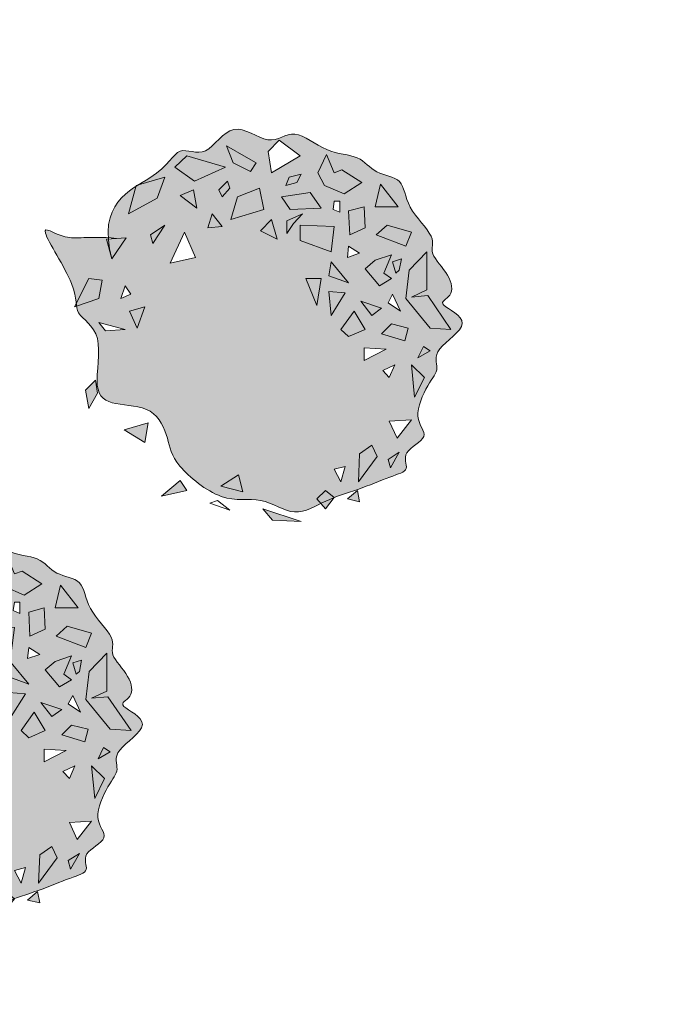
# Model space of a CAD drawing. Units: metres. Extents: x 4298.5 to 4325.2, y 2075 to 2095.8.
# Tile 24 of 35: x 4319.132 to 4320.125, y 2078.198 to 2079.73. Entities that reach past the tile are written whole.
import ezdxf

# ---------------------------------------------------------------- set-up
doc = ezdxf.new("R2010")
doc.units = ezdxf.units.M
doc.layers.add('A-ANNO-DIMS', color=2, linetype='Continuous', lineweight=18)
doc.layers.add('L-PLNT', color=94, linetype='Continuous', lineweight=13)
doc.layers.add('L-PLNT-PATT', color=116, linetype='Continuous', lineweight=13, true_color=0x13823e)
doc.styles.get("Standard").update_dxf_attribs({"font": 'arial.ttf'})
doc.dimstyles.get("Standard").update_dxf_attribs({"dimtxt": 0.18, "dimasz": 0.18, "dimexe": 0.18, "dimexo": 0.0625, "dimgap": 0.09, "dimtad": 0, "dimtih": 1, "dimtoh": 1, "dimdec": 4, "dimzin": 0, "dimdsep": 46, "dimtxsty": 'Standard', "dimcen": 0.09, "dimadec": 0, "dimazin": 0, "dimtfac": 1, "dimtdec": 4, "dimtofl": 0, "dimtmove": 0, "dimatfit": 3, "dimfxl": 1, "dimtolj": 1, "dimtzin": 0, "dimarcsym": 0})

# ---------------------------------------------------------------- blocks, each defined once
blk = doc.blocks.new('*U9')
for points in [[(-2.003, 11.656), (-1.598, 10.618), (-0.518, 10.099), (-0.181, 10.618), (-0.788, 10.964)], [(1.237, 12.003), (0.562, 11.31), (0.764, 10.013), (2.519, 11.051)], [(-4.432, 11.051), (-5.175, 10.359), (-3.96, 9.493), (-2.07, 10.359)], [(4.139, 11.137), (3.599, 10.013), (4.004, 9.234), (5.218, 8.715), (6.298, 9.407), (5.083, 10.186), (4.611, 10.013)], [(-5.782, 9.753), (-7.537, 9.234), (-8.009, 7.504), (-6.255, 8.455)], [(2.586, 9.926), (1.844, 9.753), (1.642, 9.234), (2.316, 9.407)], [(-1.935, 9.493), (-2.475, 8.974), (-2.273, 8.542), (-1.8, 9.061)], [(0.022, 9.061), (-1.328, 8.542), (-1.733, 7.157), (0.292, 7.763)], [(7.446, 9.32), (7.108, 7.936), (8.525, 7.936)], [(-4.837, 8.628), (-3.825, 7.85), (-4.027, 8.974)], [(1.372, 8.542), (3.126, 8.801), (3.801, 7.85), (1.912, 7.763)], [(4.611, 8.282), (4.544, 7.763), (4.949, 7.59), (4.949, 8.282)], [(6.433, 7.936), (5.488, 7.676), (5.556, 6.206), (6.501, 6.638)], [(-2.88, 7.504), (-3.15, 6.638), (-2.273, 6.725)], [(1.709, 6.292), (1.709, 7.071), (2.654, 7.504), (2.114, 6.898)], [(-5.782, 6.811), (-6.659, 6.206), (-6.524, 5.687)], [(0.764, 7.157), (0.089, 6.465), (1.102, 5.946)], [(2.519, 6.811), (2.519, 5.86), (4.409, 5.167), (4.611, 6.725)], [(7.851, 6.811), (7.176, 6.206), (8.998, 5.514), (9.335, 6.379)], [(-4.567, 6.379), (-5.445, 4.475), (-3.892, 4.821)], [(-8.144, 6.033), (-9.359, 5.946), (-9.022, 4.735)], [(5.488, 5.514), (5.421, 4.821), (6.163, 5.081)], [(8.12, 4.994), (7.108, 4.648), (6.501, 4.129), (7.378, 3.091), (8.12, 3.524), (7.648, 3.87)], [(10.28, 5.167), (9.2, 4.043), (8.998, 2.312), (10.482, 0.495), (11.765, 0.409), (10.348, 2.485), (9.335, 2.399), (10.28, 2.831)], [(4.409, 4.562), (4.274, 3.697), (5.488, 3.264)], [(8.728, 4.735), (8.188, 4.562), (8.39, 3.87), (8.593, 4.043)], [(-11.316, 1.793), (-9.831, 2.312), (-9.629, 3.437), (-10.439, 3.524)], [(-8.212, 3.091), (-8.482, 2.312), (-7.874, 2.572)], [(3.531, 1.88), (2.856, 3.524), (3.801, 3.524)], [(4.274, 2.745), (5.286, 2.658), (4.409, 1.274)], [(8.188, 2.572), (7.918, 2.053), (8.66, 1.534)], [(7.513, 1.707), (6.906, 1.274), (6.231, 2.139)], [(-6.997, 1.793), (-7.942, 1.534), (-7.469, 0.495)], [(5.826, 1.534), (5.016, 0.409), (5.488, -0.024), (6.501, 0.409)], [(-8.212, 0.409), (-9.426, 0.322), (-9.831, 0.841)], [(8.12, 0.755), (7.513, 0.149), (8.93, -0.283), (9.133, 0.495)], [(7.783, -0.803), (6.433, -1.495), (6.433, -0.716)], [(10.078, -0.629), (9.74, -1.322), (10.482, -0.889)], [(8.323, -1.754), (7.985, -2.533), (7.581, -2.1)], [(9.335, -1.754), (9.538, -3.744), (10.145, -2.533)], [(-10.034, -2.706), (-10.641, -3.312), (-10.439, -4.436), (-9.899, -3.485)], [(-8.279, -5.734), (-6.794, -5.302), (-6.997, -6.513)], [(9.335, -5.129), (8.458, -6.253), (7.985, -5.215)], [(6.096, -8.935), (6.163, -7.205), (6.906, -6.686), (7.243, -7.378)], [(8.053, -8.07), (8.593, -7.118), (7.918, -7.551)], [(5.286, -7.984), (4.611, -8.157), (5.016, -8.935)], [(-4.837, -8.849), (-4.432, -9.454), (-5.985, -9.801)], [(-2.34, -9.195), (-1.26, -8.503), (-0.99, -9.541)], [(4.071, -9.454), (3.531, -9.974), (4.071, -10.579), (4.611, -9.887)], [(6.028, -9.454), (5.421, -9.974), (6.163, -10.147)], [(-2.543, -10.06), (-3.015, -10.233), (-1.8, -10.666)], [(0.224, -10.579), (0.832, -11.272), (2.586, -11.358)]]:
    blk.add_lwpolyline(points, close=True)
blk = doc.blocks.new('*D47')
at = {"layer": 'A-ANNO-DIMS', "color": 0, "lineweight": -2, "transparency": 16777216}
for p, q in [((4300.4306, 2084.4956), (4300.4306, 2074.9896)), ((4322.8106, 2084.4956), (4322.8106, 2074.9896)), ((4300.6106, 2075.1696), (4311.2252, 2075.1696)), ((4322.6306, 2075.1696), (4312.016, 2075.1696))]:
    blk.add_line(p, q, dxfattribs=at)
at = {"layer": 'A-ANNO-DIMS', "color": 0, "transparency": 16777216}
for points in [[(4300.6106, 2075.1996), (4300.6106, 2075.1396), (4300.4306, 2075.1696)], [(4322.6306, 2075.1996), (4322.6306, 2075.1396), (4322.8106, 2075.1696)]]:
    blk.add_solid(points, dxfattribs=at)
at = {"layer": 'Defpoints', "color": 0, "transparency": 16777216}
for p in [(4300.4306, 2084.5581), (4322.8106, 2084.5581), (4322.8106, 2075.1696)]:
    blk.add_point(p, dxfattribs=at)
at = {"layer": 'A-ANNO-DIMS', "color": 0, "transparency": 16777216, "insert": (4311.6206, 2075.1696), "char_height": 0.18, "attachment_point": 5}
blk.add_mtext('\\A1;22.38', dxfattribs=at)
blk = doc.blocks.new('*D48')
at = {"layer": 'A-ANNO-DIMS', "color": 0, "lineweight": -2, "transparency": 16777216}
for p, q in [((4310.1831, 2094.4781), (4324.7671, 2094.4781)), ((4324.5871, 2094.2981), (4324.5871, 2085.585)), ((4324.5871, 2076.5081), (4324.5871, 2085.2212)), ((4316.8731, 2076.3281), (4324.7671, 2076.3281))]:
    blk.add_line(p, q, dxfattribs=at)
at = {"layer": 'A-ANNO-DIMS', "color": 0, "transparency": 16777216}
for points in [[(4324.5571, 2094.2981), (4324.6171, 2094.2981), (4324.5871, 2094.4781)], [(4324.5571, 2076.5081), (4324.6171, 2076.5081), (4324.5871, 2076.3281)]]:
    blk.add_solid(points, dxfattribs=at)
at = {"layer": 'Defpoints', "color": 0, "transparency": 16777216}
for p in [(4310.1206, 2094.4781), (4316.8106, 2076.3281), (4324.5871, 2076.3281)]:
    blk.add_point(p, dxfattribs=at)
at = {"layer": 'A-ANNO-DIMS', "color": 0, "transparency": 16777216, "insert": (4324.5871, 2085.4031), "char_height": 0.18, "attachment_point": 5}
blk.add_mtext('\\A1;18.15', dxfattribs=at)
blk = doc.blocks.new('*D79')
at = {"layer": 'A-ANNO-DIMS', "color": 0, "lineweight": -2, "transparency": 16777216}
for p, q in [((4313.4743, 2079.7393), (4313.4743, 2079.9193)), ((4313.3843, 2079.8293), (4313.5643, 2079.8293)), ((4320.4622, 2076.981), (4318.0084, 2077.9812)), ((4320.6422, 2076.981), (4320.4622, 2076.981))]:
    blk.add_line(p, q, dxfattribs=at)
at = {"layer": 'A-ANNO-DIMS', "color": 0, "transparency": 16777216}
blk.add_solid([(4318.0197, 2078.009), (4317.9971, 2077.9534), (4317.8417, 2078.0491)], dxfattribs=at)
at = {"layer": 'Defpoints', "color": 0, "transparency": 16777216}
for p in [(4313.4743, 2079.8293), (4317.8417, 2078.0491)]:
    blk.add_point(p, dxfattribs=at)
at = {"layer": 'A-ANNO-DIMS', "color": 0, "transparency": 16777216, "insert": (4321.3169, 2076.981), "char_height": 0.18, "attachment_point": 5}
blk.add_mtext('\\A1;2X R4.716', dxfattribs=at)

msp = doc.modelspace()

# ---------------------------------------------------------------- hatches: boundary and pattern name
at = {"layer": 'L-PLNT-PATT'}
h = msp.add_hatch(color=256, dxfattribs=at)
h.dxf.hatch_style = 1
edge = h.paths.add_edge_path()
edge.add_spline(control_points=[(4319.6008, 2078.9772), (4319.6034, 2078.9785), (4319.622, 2078.9878), (4319.6578, 2078.9976), (4319.7123, 2079.0208), (4319.7417, 2079.0284), (4319.723, 2079.0569), (4319.7755, 2079.0811), (4319.7418, 2079.1074), (4319.7688, 2079.1671), (4319.7876, 2079.1866), (4319.7709, 2079.2151), (4319.8452, 2079.26), (4319.7752, 2079.2895), (4319.8079, 2079.2972), (4319.8039, 2079.3323), (4319.7658, 2079.3689), (4319.7844, 2079.3883), (4319.7313, 2079.4393), (4319.7313, 2079.4853), (4319.6835, 2079.4887), (4319.663, 2079.5206), (4319.6098, 2079.5206), (4319.5575, 2079.5659), (4319.5227, 2079.5288), (4319.462, 2079.5797), (4319.4221, 2079.5096), (4319.3776, 2079.5396), (4319.3632, 2079.5002), (4319.3229, 2079.4772), (4319.3166, 2079.4732)], knot_values=[0.818571, 0.818571, 0.818571, 0.818571, 0.97924, 1.97924, 2.97924, 3.97924, 4.97924, 5.97924, 6.97924, 7.97924, 8.97924, 9.97924, 10.97924, 11.97924, 12.97924, 13.97924, 14.97924, 15.97924, 16.97924, 17.97924, 18.97924, 19.97924, 20.97924, 21.97924, 22.97924, 23.97924, 24.97924, 25.97924, 26.97924, 27.16067, 27.16067, 27.16067, 27.16067], degree=3, periodic=0)
edge.add_line((4319.3166, 2079.4732), (4319.3578, 2079.4854))
edge.add_line((4319.3578, 2079.4854), (4319.3458, 2079.4524))
edge.add_line((4319.3458, 2079.4524), (4319.3013, 2079.4283))
edge.add_line((4319.3013, 2079.4283), (4319.3129, 2079.4709))
edge.add_spline(control_points=[(4319.3129, 2079.4709), (4319.2902, 2079.4562), (4319.267, 2079.4353), (4319.2697, 2079.3909)], knot_values=[0.141368, 0.141368, 0.141368, 0.141368, 0.783694, 0.783694, 0.783694, 0.783694], degree=3, periodic=0)
edge.add_spline(control_points=[(4319.2697, 2079.3909), (4319.2737, 2079.3906), (4319.2779, 2079.3903), (4319.2824, 2079.3898)], knot_values=[40.901028, 40.901028, 40.901028, 40.901028, 41, 41, 41, 41], degree=3, periodic=0)
edge.add_line((4319.2824, 2079.3898), (4319.2978, 2079.3909))
edge.add_line((4319.2978, 2079.3909), (4319.2755, 2079.358))
edge.add_line((4319.2755, 2079.358), (4319.267, 2079.3887))
edge.add_line((4319.267, 2079.3887), (4319.2698, 2079.3889))
edge.add_spline(control_points=[(4319.2698, 2079.3889), (4319.2698, 2079.3896), (4319.2697, 2079.3902), (4319.2697, 2079.3909)], knot_values=[0.13204, 0.13204, 0.13204, 0.13204, 0.141368, 0.141368, 0.141368, 0.141368], degree=3, periodic=0)
edge.add_spline(control_points=[(4319.2697, 2079.3909), (4319.2335, 2079.3932), (4319.2019, 2079.3834), (4319.1498, 2079.4253), (4319.2169, 2079.3228), (4319.2192, 2079.2959), (4319.2199, 2079.2885)], knot_values=[37.439141, 37.439141, 37.439141, 37.439141, 38.340169, 39.340169, 40.340169, 40.901028, 40.901028, 40.901028, 40.901028], degree=3, periodic=0)
edge.add_line((4319.2199, 2079.2885), (4319.2395, 2079.3272))
edge.add_line((4319.2395, 2079.3272), (4319.2601, 2079.325))
edge.add_line((4319.2601, 2079.325), (4319.255, 2079.2964))
edge.add_line((4319.255, 2079.2964), (4319.2204, 2079.2843))
edge.add_spline(control_points=[(4319.2204, 2079.2843), (4319.2208, 2079.2804), (4319.2239, 2079.2668), (4319.2653, 2079.2459), (4319.2438, 2079.1486), (4319.2761, 2079.1297), (4319.3423, 2079.1297), (4319.365, 2079.076), (4319.3685, 2079.0405), (4319.4495, 2078.9745), (4319.5078, 2078.9912), (4319.5582, 2078.9544), (4319.5874, 2078.9703), (4319.6008, 2078.9772)], knot_values=[27.16067, 27.16067, 27.16067, 27.16067, 27.490087, 28.490087, 29.490087, 30.490087, 31.490087, 32.490087, 33.490087, 34.490087, 35.490087, 36.490087, 37.329418, 37.329418, 37.329418, 37.329418], degree=3, periodic=0)
edge.add_line((4319.6008, 2078.9772), (4319.5944, 2078.9843))
edge.add_line((4319.5944, 2078.9843), (4319.6081, 2078.9976))
edge.add_line((4319.6081, 2078.9976), (4319.6218, 2078.9865))
h.paths.add_polyline_path([(4319.5772, 2079.3272), (4319.6012, 2079.3272), (4319.5944, 2079.2854)], flags=16)
h.paths.add_polyline_path([(4319.6133, 2079.3074), (4319.639, 2079.3052), (4319.6167, 2079.27)], flags=16)
h.paths.add_polyline_path([(4319.4058, 2079.3601), (4319.3664, 2079.3514), (4319.3887, 2079.3997)], flags=16)
h.paths.add_polyline_path([(4319.5327, 2079.3887), (4319.507, 2079.4019), (4319.5241, 2079.4195)], flags=16)
h.paths.add_polyline_path([(4319.6133, 2079.3316), (4319.6167, 2079.3536), (4319.6441, 2079.3206)], flags=16)
h.paths.add_polyline_path([(4319.6321, 2079.2481), (4319.6527, 2079.2766), (4319.6698, 2079.2481), (4319.6441, 2079.2371)], flags=16)
h.paths.add_polyline_path([(4319.5687, 2079.3865), (4319.5687, 2079.4107), (4319.6218, 2079.4085), (4319.6167, 2079.3689)], flags=16)
h.paths.add_polyline_path([(4319.5481, 2079.3975), (4319.5481, 2079.4173), (4319.5721, 2079.4283), (4319.5584, 2079.4129)], flags=16)
h.paths.add_polyline_path([(4319.447, 2079.4085), (4319.4247, 2079.4063), (4319.4315, 2079.4283)], flags=16)
h.paths.add_polyline_path([(4319.4607, 2079.4195), (4319.471, 2079.4547), (4319.5053, 2079.4678), (4319.5121, 2079.4349)], flags=16)
h.paths.add_polyline_path([(4319.327, 2079.2832), (4319.315, 2079.2503), (4319.303, 2079.2766)], flags=16)
h.paths.add_polyline_path([(4319.663, 2079.292), (4319.6955, 2079.281), (4319.6801, 2079.27)], flags=16)
h.paths.add_polyline_path([(4319.6424, 2079.3601), (4319.6441, 2079.3777), (4319.6612, 2079.3667)], flags=16)
h.paths.add_polyline_path([(4319.5533, 2079.4349), (4319.5395, 2079.4547), (4319.5841, 2079.4612), (4319.6012, 2079.4371)], flags=16)
h.paths.add_polyline_path([(4319.6681, 2079.2195), (4319.7024, 2079.2173), (4319.6681, 2079.1997)], flags=16)
h.paths.add_polyline_path([(4319.3047, 2079.303), (4319.2893, 2079.2964), (4319.2961, 2079.3162)], flags=16)
h.paths.add_polyline_path([(4319.4075, 2079.4371), (4319.3818, 2079.4568), (4319.4024, 2079.4656)], flags=16)
h.paths.add_polyline_path([(4319.339, 2079.3821), (4319.3356, 2079.3953), (4319.3578, 2079.4107)], flags=16)
h.paths.add_polyline_path([(4319.447, 2079.4547), (4319.4418, 2079.4656), (4319.4555, 2079.4788), (4319.459, 2079.4678)], flags=16)
h.paths.add_polyline_path([(4319.6698, 2079.3426), (4319.6852, 2079.3557), (4319.7109, 2079.3645), (4319.699, 2079.336), (4319.7109, 2079.3272), (4319.6921, 2079.3162)], flags=16)
h.paths.add_polyline_path([(4319.2961, 2079.2481), (4319.2653, 2079.2459), (4319.255, 2079.259)], flags=16)
h.paths.add_polyline_path([(4319.6458, 2079.3953), (4319.6441, 2079.4327), (4319.6681, 2079.4393), (4319.6698, 2079.4063)], flags=16)
h.paths.add_polyline_path([(4319.6955, 2079.2415), (4319.7109, 2079.2569), (4319.7367, 2079.2503), (4319.7315, 2079.2305)], flags=16)
h.paths.add_polyline_path([(4319.6201, 2079.4349), (4319.6218, 2079.448), (4319.6304, 2079.448), (4319.6304, 2079.4305)], flags=16)
h.paths.add_polyline_path([(4319.5464, 2079.4722), (4319.5515, 2079.4854), (4319.5704, 2079.4898), (4319.5635, 2079.4766)], flags=16)
h.paths.add_polyline_path([(4319.7058, 2079.2898), (4319.7127, 2079.303), (4319.7247, 2079.2766)], flags=16)
h.paths.add_polyline_path([(4319.6973, 2079.1843), (4319.7161, 2079.1931), (4319.7075, 2079.1733)], flags=16)
h.paths.add_polyline_path([(4319.4915, 2079.4942), (4319.4641, 2079.5074), (4319.4538, 2079.5337), (4319.4847, 2079.5162), (4319.5001, 2079.5074)], flags=16)
h.paths.add_polyline_path([(4319.5241, 2079.492), (4319.519, 2079.525), (4319.5361, 2079.5426), (4319.5687, 2079.5184)], flags=16)
h.paths.add_polyline_path([(4319.4041, 2079.4788), (4319.3733, 2079.5008), (4319.3921, 2079.5184), (4319.4521, 2079.5008)], flags=16)
h.paths.add_polyline_path([(4319.687, 2079.3953), (4319.7041, 2079.4107), (4319.7418, 2079.3997), (4319.7332, 2079.3777)], flags=16)
h.paths.add_polyline_path([(4319.6064, 2079.4722), (4319.5961, 2079.492), (4319.6098, 2079.5206), (4319.6218, 2079.492), (4319.6338, 2079.4964), (4319.6647, 2079.4766), (4319.6372, 2079.459)], flags=16)
h.paths.add_polyline_path([(4319.7178, 2079.336), (4319.7127, 2079.3536), (4319.7264, 2079.358), (4319.723, 2079.3404)], flags=16)
h.paths.add_polyline_path([(4319.7332, 2079.2964), (4319.7384, 2079.3404), (4319.7658, 2079.3689), (4319.7658, 2079.3096), (4319.7418, 2079.2986), (4319.7675, 2079.3008), (4319.8035, 2079.2481), (4319.7709, 2079.2503)], flags=16)
h.paths.add_polyline_path([(4319.4727, 2079.0217), (4319.4796, 2078.9953), (4319.4453, 2079.0041)], flags=16)
h.paths.add_polyline_path([(4319.6852, 2079.4393), (4319.6938, 2079.4744), (4319.7212, 2079.4393)], flags=16)
h.paths.add_polyline_path([(4319.7418, 2079.1931), (4319.7624, 2079.1733), (4319.747, 2079.1426)], flags=16)
h.paths.add_polyline_path([(4319.7521, 2079.2041), (4319.7607, 2079.2217), (4319.7709, 2079.2151)], flags=16)
h.paths.add_polyline_path([(4319.6218, 2079.0305), (4319.639, 2079.0349), (4319.6321, 2079.0107)], flags=16)
h.paths.add_polyline_path([(4319.7075, 2079.1052), (4319.7418, 2079.1074), (4319.7195, 2079.0789)], flags=16)
h.paths.add_polyline_path([(4319.6612, 2079.0547), (4319.6801, 2079.0679), (4319.6887, 2079.0503), (4319.6595, 2079.0107)], flags=16)
h.paths.add_polyline_path([(4319.7058, 2079.0459), (4319.723, 2079.0569), (4319.7092, 2079.0327)], flags=16)
h = msp.add_hatch(color=256, dxfattribs=at)
h.dxf.hatch_style = 1
h.paths.add_polyline_path([(4319.6167, 2079.3689), (4319.6218, 2079.4085), (4319.5687, 2079.4107), (4319.5687, 2079.3865)])
h.paths.add_polyline_path([(4319.663, 2079.292), (4319.6801, 2079.27), (4319.6955, 2079.281)])
h.paths.add_polyline_path([(4319.6441, 2079.4327), (4319.6458, 2079.3953), (4319.6698, 2079.4063), (4319.6681, 2079.4393)])
h.paths.add_polyline_path([(4319.6647, 2079.4766), (4319.6338, 2079.4964), (4319.6218, 2079.492), (4319.6098, 2079.5206), (4319.5961, 2079.492), (4319.6064, 2079.4722), (4319.6372, 2079.459)])
h.paths.add_polyline_path([(4319.5104, 2078.969), (4319.5258, 2078.9514), (4319.5704, 2078.9492)])
h.paths.add_polyline_path([(4319.4915, 2079.4942), (4319.5001, 2079.5074), (4319.4847, 2079.5162), (4319.4538, 2079.5337), (4319.4641, 2079.5074)])
h.paths.add_polyline_path([(4319.3921, 2079.5184), (4319.3733, 2079.5008), (4319.4041, 2079.4788), (4319.4521, 2079.5008)])
h.paths.add_polyline_path([(4319.471, 2079.4547), (4319.4607, 2079.4195), (4319.5121, 2079.4349), (4319.5053, 2079.4678)])
h.paths.add_polyline_path([(4319.459, 2079.4678), (4319.4555, 2079.4788), (4319.4418, 2079.4656), (4319.447, 2079.4547)])
h.paths.add_polyline_path([(4319.4315, 2079.4283), (4319.4247, 2079.4063), (4319.447, 2079.4085)])
h.paths.add_polyline_path([(4319.4075, 2079.4371), (4319.4024, 2079.4656), (4319.3818, 2079.4568)])
h.paths.add_polyline_path([(4319.3133, 2079.4722), (4319.3013, 2079.4283), (4319.3458, 2079.4524), (4319.3578, 2079.4854)])
h.paths.add_polyline_path([(4319.3578, 2079.4107), (4319.3356, 2079.3953), (4319.339, 2079.3821)])
h.paths.add_polyline_path([(4319.267, 2079.3887), (4319.2755, 2079.358), (4319.2978, 2079.3909)])
h.paths.add_polyline_path([(4319.2173, 2079.2832), (4319.255, 2079.2964), (4319.2601, 2079.325), (4319.2395, 2079.3272)])
h.paths.add_polyline_path([(4319.327, 2079.2832), (4319.303, 2079.2766), (4319.315, 2079.2503)])
h.paths.add_polyline_path([(4319.2533, 2079.1492), (4319.2498, 2079.169), (4319.2344, 2079.1536), (4319.2395, 2079.125)])
h.paths.add_polyline_path([(4319.3321, 2079.103), (4319.2944, 2079.092), (4319.327, 2079.0723)])
h.paths.add_polyline_path([(4319.3527, 2078.9887), (4319.3921, 2078.9976), (4319.3818, 2079.0129)])
h.paths.add_polyline_path([(4319.4727, 2079.0217), (4319.4453, 2079.0041), (4319.4796, 2078.9953)])
h.paths.add_polyline_path([(4319.6081, 2078.9976), (4319.5944, 2078.9843), (4319.6081, 2078.969), (4319.6218, 2078.9866)])
h.paths.add_polyline_path([(4319.6887, 2079.0503), (4319.6801, 2079.0679), (4319.6612, 2079.0547), (4319.6595, 2079.0107)])
h.paths.add_polyline_path([(4319.6578, 2078.9976), (4319.6424, 2078.9843), (4319.6612, 2078.98)])
h.paths.add_polyline_path([(4319.7058, 2079.0459), (4319.7092, 2079.0327), (4319.723, 2079.0569)])
h.paths.add_polyline_path([(4319.747, 2079.1426), (4319.7624, 2079.1733), (4319.7418, 2079.1931)])
h.paths.add_polyline_path([(4319.6321, 2079.2481), (4319.6441, 2079.2371), (4319.6698, 2079.2481), (4319.6527, 2079.2766)])
h.paths.add_polyline_path([(4319.7709, 2079.2503), (4319.8035, 2079.2481), (4319.7675, 2079.3008), (4319.7418, 2079.2986), (4319.7658, 2079.3096), (4319.7658, 2079.3689), (4319.7384, 2079.3404), (4319.7332, 2079.2964)])
h.paths.add_polyline_path([(4319.7109, 2079.2569), (4319.6955, 2079.2415), (4319.7315, 2079.2305), (4319.7367, 2079.2503)])
h.paths.add_polyline_path([(4319.7709, 2079.2151), (4319.7607, 2079.2217), (4319.7521, 2079.2041)])
h.paths.add_polyline_path([(4319.7109, 2079.3645), (4319.6852, 2079.3557), (4319.6698, 2079.3426), (4319.6921, 2079.3162), (4319.7109, 2079.3272), (4319.699, 2079.336)])
h.paths.add_polyline_path([(4319.7127, 2079.3536), (4319.7178, 2079.336), (4319.723, 2079.3404), (4319.7264, 2079.358)])
h.paths.add_polyline_path([(4319.7332, 2079.3777), (4319.7418, 2079.3997), (4319.7041, 2079.4107), (4319.687, 2079.3953)])
h.paths.add_polyline_path([(4319.6441, 2079.3206), (4319.6167, 2079.3536), (4319.6133, 2079.3316)])
h.paths.add_polyline_path([(4319.6012, 2079.3272), (4319.5772, 2079.3272), (4319.5944, 2079.2854)])
h.paths.add_polyline_path([(4319.639, 2079.3052), (4319.6133, 2079.3074), (4319.6167, 2079.27)])
h.paths.add_polyline_path([(4319.6012, 2079.4371), (4319.5841, 2079.4612), (4319.5395, 2079.4547), (4319.5533, 2079.4349)])
h.paths.add_polyline_path([(4319.5584, 2079.4129), (4319.5721, 2079.4283), (4319.5481, 2079.4173), (4319.5481, 2079.3975)])
h.paths.add_polyline_path([(4319.5241, 2079.4195), (4319.507, 2079.4019), (4319.5327, 2079.3887)])
h.paths.add_polyline_path([(4319.5635, 2079.4766), (4319.5704, 2079.4898), (4319.5515, 2079.4854), (4319.5464, 2079.4722)])
h.paths.add_polyline_path([(4319.6938, 2079.4744), (4319.6852, 2079.4393), (4319.7212, 2079.4393)])
h = msp.add_hatch(color=256, dxfattribs=at)
h.dxf.hatch_style = 1
edge = h.paths.add_edge_path()
edge.add_spline(control_points=[(4319.1026, 2078.3528), (4319.1051, 2078.3541), (4319.1238, 2078.3634), (4319.1596, 2078.3732), (4319.2141, 2078.3964), (4319.2435, 2078.4041), (4319.2247, 2078.4325), (4319.2773, 2078.4567), (4319.2436, 2078.483), (4319.2706, 2078.5428), (4319.2893, 2078.5622), (4319.2727, 2078.5907), (4319.3469, 2078.6356), (4319.277, 2078.6652), (4319.3097, 2078.6728), (4319.3057, 2078.7079), (4319.2676, 2078.7446), (4319.2862, 2078.7639), (4319.2331, 2078.8149), (4319.2331, 2078.8609), (4319.1852, 2078.8643), (4319.1648, 2078.8962), (4319.1116, 2078.8962), (4319.0593, 2078.9415), (4319.0245, 2078.9044), (4318.9638, 2078.9553), (4318.9239, 2078.8852), (4318.8793, 2078.9152), (4318.865, 2078.8758), (4318.8247, 2078.8528), (4318.8183, 2078.8488)], knot_values=[0.818571, 0.818571, 0.818571, 0.818571, 0.97924, 1.97924, 2.97924, 3.97924, 4.97924, 5.97924, 6.97924, 7.97924, 8.97924, 9.97924, 10.97924, 11.97924, 12.97924, 13.97924, 14.97924, 15.97924, 16.97924, 17.97924, 18.97924, 19.97924, 20.97924, 21.97924, 22.97924, 23.97924, 24.97924, 25.97924, 26.97924, 27.16067, 27.16067, 27.16067, 27.16067], degree=3, periodic=0)
edge.add_line((4318.8183, 2078.8488), (4318.8596, 2078.861))
edge.add_line((4318.8596, 2078.861), (4318.8476, 2078.8281))
edge.add_line((4318.8476, 2078.8281), (4318.803, 2078.8039))
edge.add_line((4318.803, 2078.8039), (4318.8147, 2078.8465))
edge.add_spline(control_points=[(4318.8147, 2078.8465), (4318.792, 2078.8318), (4318.7687, 2078.8109), (4318.7714, 2078.7665)], knot_values=[0.141368, 0.141368, 0.141368, 0.141368, 0.783694, 0.783694, 0.783694, 0.783694], degree=3, periodic=0)
edge.add_spline(control_points=[(4318.7714, 2078.7665), (4318.7754, 2078.7662), (4318.7797, 2078.7659), (4318.7842, 2078.7654)], knot_values=[40.901028, 40.901028, 40.901028, 40.901028, 41, 41, 41, 41], degree=3, periodic=0)
edge.add_line((4318.7842, 2078.7654), (4318.7996, 2078.7665))
edge.add_line((4318.7996, 2078.7665), (4318.7773, 2078.7336))
edge.add_line((4318.7773, 2078.7336), (4318.7688, 2078.7643))
edge.add_line((4318.7688, 2078.7643), (4318.7716, 2078.7645))
edge.add_spline(control_points=[(4318.7716, 2078.7645), (4318.7715, 2078.7652), (4318.7715, 2078.7658), (4318.7714, 2078.7665)], knot_values=[0.13204, 0.13204, 0.13204, 0.13204, 0.141368, 0.141368, 0.141368, 0.141368], degree=3, periodic=0)
edge.add_spline(control_points=[(4318.7714, 2078.7665), (4318.7352, 2078.7688), (4318.7036, 2078.759), (4318.6516, 2078.801), (4318.7187, 2078.6984), (4318.721, 2078.6716), (4318.7217, 2078.6641)], knot_values=[37.439141, 37.439141, 37.439141, 37.439141, 38.340169, 39.340169, 40.340169, 40.901028, 40.901028, 40.901028, 40.901028], degree=3, periodic=0)
edge.add_line((4318.7217, 2078.6641), (4318.7413, 2078.7028))
edge.add_line((4318.7413, 2078.7028), (4318.7619, 2078.7006))
edge.add_line((4318.7619, 2078.7006), (4318.7568, 2078.672))
edge.add_line((4318.7568, 2078.672), (4318.7221, 2078.6599))
edge.add_spline(control_points=[(4318.7221, 2078.6599), (4318.7226, 2078.656), (4318.7257, 2078.6424), (4318.767, 2078.6215), (4318.7456, 2078.5242), (4318.7778, 2078.5054), (4318.8441, 2078.5054), (4318.8668, 2078.4516), (4318.8703, 2078.4162), (4318.9513, 2078.3501), (4319.0096, 2078.3669), (4319.06, 2078.33), (4319.0891, 2078.3459), (4319.1026, 2078.3528)], knot_values=[27.16067, 27.16067, 27.16067, 27.16067, 27.490087, 28.490087, 29.490087, 30.490087, 31.490087, 32.490087, 33.490087, 34.490087, 35.490087, 36.490087, 37.329418, 37.329418, 37.329418, 37.329418], degree=3, periodic=0)
edge.add_line((4319.1026, 2078.3528), (4319.0962, 2078.36))
edge.add_line((4319.0962, 2078.36), (4319.1099, 2078.3732))
edge.add_line((4319.1099, 2078.3732), (4319.1236, 2078.3622))
h.paths.add_polyline_path([(4319.079, 2078.7028), (4319.103, 2078.7028), (4319.0962, 2078.6611)], flags=16)
h.paths.add_polyline_path([(4319.115, 2078.683), (4319.1407, 2078.6808), (4319.1185, 2078.6457)], flags=16)
h.paths.add_polyline_path([(4318.9076, 2078.7358), (4318.8682, 2078.727), (4318.8905, 2078.7753)], flags=16)
h.paths.add_polyline_path([(4319.0345, 2078.7643), (4319.0087, 2078.7775), (4319.0259, 2078.7951)], flags=16)
h.paths.add_polyline_path([(4319.115, 2078.7072), (4319.1185, 2078.7292), (4319.1459, 2078.6962)], flags=16)
h.paths.add_polyline_path([(4319.1339, 2078.6237), (4319.1544, 2078.6523), (4319.1716, 2078.6237), (4319.1459, 2078.6127)], flags=16)
h.paths.add_polyline_path([(4319.0705, 2078.7622), (4319.0705, 2078.7863), (4319.1236, 2078.7841), (4319.1185, 2078.7446)], flags=16)
h.paths.add_polyline_path([(4319.0499, 2078.7731), (4319.0499, 2078.7929), (4319.0739, 2078.8039), (4319.0602, 2078.7885)], flags=16)
h.paths.add_polyline_path([(4318.9487, 2078.7841), (4318.9265, 2078.7819), (4318.9333, 2078.8039)], flags=16)
h.paths.add_polyline_path([(4318.9625, 2078.7951), (4318.9727, 2078.8303), (4319.007, 2078.8435), (4319.0139, 2078.8105)], flags=16)
h.paths.add_polyline_path([(4318.8287, 2078.6589), (4318.8168, 2078.6259), (4318.8047, 2078.6523)], flags=16)
h.paths.add_polyline_path([(4319.1647, 2078.6676), (4319.1973, 2078.6567), (4319.1819, 2078.6457)], flags=16)
h.paths.add_polyline_path([(4319.1442, 2078.7358), (4319.1459, 2078.7534), (4319.163, 2078.7424)], flags=16)
h.paths.add_polyline_path([(4319.055, 2078.8105), (4319.0413, 2078.8303), (4319.0859, 2078.8369), (4319.103, 2078.8127)], flags=16)
h.paths.add_polyline_path([(4319.1699, 2078.5951), (4319.2042, 2078.5929), (4319.1699, 2078.5753)], flags=16)
h.paths.add_polyline_path([(4318.8065, 2078.6786), (4318.791, 2078.672), (4318.7979, 2078.6918)], flags=16)
h.paths.add_polyline_path([(4318.9093, 2078.8127), (4318.8836, 2078.8325), (4318.9042, 2078.8412)], flags=16)
h.paths.add_polyline_path([(4318.8408, 2078.7578), (4318.8373, 2078.7709), (4318.8596, 2078.7863)], flags=16)
h.paths.add_polyline_path([(4318.9487, 2078.8303), (4318.9436, 2078.8412), (4318.9573, 2078.8544), (4318.9607, 2078.8435)], flags=16)
h.paths.add_polyline_path([(4319.1716, 2078.7182), (4319.187, 2078.7314), (4319.2127, 2078.7402), (4319.2007, 2078.7116), (4319.2127, 2078.7028), (4319.1939, 2078.6918)], flags=16)
h.paths.add_polyline_path([(4318.7979, 2078.6237), (4318.767, 2078.6215), (4318.7568, 2078.6347)], flags=16)
h.paths.add_polyline_path([(4319.1476, 2078.7709), (4319.1459, 2078.8083), (4319.1699, 2078.8149), (4319.1716, 2078.7819)], flags=16)
h.paths.add_polyline_path([(4319.1973, 2078.6171), (4319.2127, 2078.6325), (4319.2384, 2078.6259), (4319.2333, 2078.6061)], flags=16)
h.paths.add_polyline_path([(4319.1219, 2078.8105), (4319.1236, 2078.8237), (4319.1322, 2078.8237), (4319.1322, 2078.8061)], flags=16)
h.paths.add_polyline_path([(4319.0482, 2078.8479), (4319.0533, 2078.861), (4319.0722, 2078.8654), (4319.0653, 2078.8522)], flags=16)
h.paths.add_polyline_path([(4319.2076, 2078.6655), (4319.2144, 2078.6786), (4319.2264, 2078.6523)], flags=16)
h.paths.add_polyline_path([(4319.199, 2078.56), (4319.2179, 2078.5688), (4319.2093, 2078.549)], flags=16)
h.paths.add_polyline_path([(4318.9933, 2078.8698), (4318.9659, 2078.883), (4318.9556, 2078.9094), (4318.9865, 2078.8918), (4319.0019, 2078.883)], flags=16)
h.paths.add_polyline_path([(4319.0259, 2078.8676), (4319.0207, 2078.9006), (4319.0379, 2078.9182), (4319.0705, 2078.894)], flags=16)
h.paths.add_polyline_path([(4318.9059, 2078.8544), (4318.875, 2078.8764), (4318.8939, 2078.894), (4318.9539, 2078.8764)], flags=16)
h.paths.add_polyline_path([(4319.1887, 2078.7709), (4319.2059, 2078.7863), (4319.2436, 2078.7753), (4319.235, 2078.7534)], flags=16)
h.paths.add_polyline_path([(4319.1082, 2078.8479), (4319.0979, 2078.8676), (4319.1116, 2078.8962), (4319.1236, 2078.8676), (4319.1356, 2078.872), (4319.1664, 2078.8522), (4319.139, 2078.8347)], flags=16)
h.paths.add_polyline_path([(4319.2196, 2078.7116), (4319.2144, 2078.7292), (4319.2282, 2078.7336), (4319.2247, 2078.716)], flags=16)
h.paths.add_polyline_path([(4319.235, 2078.672), (4319.2401, 2078.716), (4319.2676, 2078.7446), (4319.2676, 2078.6852), (4319.2436, 2078.6742), (4319.2693, 2078.6764), (4319.3053, 2078.6237), (4319.2727, 2078.6259)], flags=16)
h.paths.add_polyline_path([(4318.9745, 2078.3973), (4318.9813, 2078.371), (4318.947, 2078.3798)], flags=16)
h.paths.add_polyline_path([(4319.187, 2078.8149), (4319.1956, 2078.85), (4319.223, 2078.8149)], flags=16)
h.paths.add_polyline_path([(4319.2436, 2078.5688), (4319.2642, 2078.549), (4319.2487, 2078.5182)], flags=16)
h.paths.add_polyline_path([(4319.2539, 2078.5797), (4319.2625, 2078.5973), (4319.2727, 2078.5907)], flags=16)
h.paths.add_polyline_path([(4319.1236, 2078.4061), (4319.1407, 2078.4105), (4319.1339, 2078.3864)], flags=16)
h.paths.add_polyline_path([(4319.2093, 2078.4808), (4319.2436, 2078.483), (4319.2213, 2078.4545)], flags=16)
h.paths.add_polyline_path([(4319.163, 2078.4303), (4319.1819, 2078.4435), (4319.1904, 2078.4259), (4319.1613, 2078.3864)], flags=16)
h.paths.add_polyline_path([(4319.2076, 2078.4215), (4319.2247, 2078.4325), (4319.211, 2078.4083)], flags=16)
h = msp.add_hatch(color=256, dxfattribs=at)
h.dxf.hatch_style = 1
h.paths.add_polyline_path([(4319.1185, 2078.7446), (4319.1236, 2078.7841), (4319.0705, 2078.7863), (4319.0705, 2078.7622)])
h.paths.add_polyline_path([(4319.1647, 2078.6676), (4319.1819, 2078.6457), (4319.1973, 2078.6567)])
h.paths.add_polyline_path([(4319.1459, 2078.8083), (4319.1476, 2078.7709), (4319.1716, 2078.7819), (4319.1699, 2078.8149)])
h.paths.add_polyline_path([(4319.1664, 2078.8522), (4319.1356, 2078.872), (4319.1236, 2078.8676), (4319.1116, 2078.8962), (4319.0979, 2078.8676), (4319.1082, 2078.8479), (4319.139, 2078.8347)])
h.paths.add_polyline_path([(4319.0122, 2078.3446), (4319.0276, 2078.327), (4319.0722, 2078.3248)])
h.paths.add_polyline_path([(4318.9933, 2078.8698), (4319.0019, 2078.883), (4318.9865, 2078.8918), (4318.9556, 2078.9094), (4318.9659, 2078.883)])
h.paths.add_polyline_path([(4318.8939, 2078.894), (4318.875, 2078.8764), (4318.9059, 2078.8544), (4318.9539, 2078.8764)])
h.paths.add_polyline_path([(4318.9727, 2078.8303), (4318.9625, 2078.7951), (4319.0139, 2078.8105), (4319.007, 2078.8435)])
h.paths.add_polyline_path([(4318.9607, 2078.8435), (4318.9573, 2078.8544), (4318.9436, 2078.8412), (4318.9487, 2078.8303)])
h.paths.add_polyline_path([(4318.9333, 2078.8039), (4318.9265, 2078.7819), (4318.9487, 2078.7841)])
h.paths.add_polyline_path([(4318.9093, 2078.8127), (4318.9042, 2078.8412), (4318.8836, 2078.8325)])
h.paths.add_polyline_path([(4318.815, 2078.8479), (4318.803, 2078.8039), (4318.8476, 2078.8281), (4318.8596, 2078.861)])
h.paths.add_polyline_path([(4318.8596, 2078.7863), (4318.8373, 2078.7709), (4318.8408, 2078.7578)])
h.paths.add_polyline_path([(4318.7688, 2078.7643), (4318.7773, 2078.7336), (4318.7996, 2078.7665)])
h.paths.add_polyline_path([(4318.719, 2078.6589), (4318.7568, 2078.672), (4318.7619, 2078.7006), (4318.7413, 2078.7028)])
h.paths.add_polyline_path([(4318.8287, 2078.6589), (4318.8047, 2078.6523), (4318.8168, 2078.6259)])
h.paths.add_polyline_path([(4318.755, 2078.5248), (4318.7516, 2078.5446), (4318.7362, 2078.5292), (4318.7413, 2078.5006)])
h.paths.add_polyline_path([(4318.8339, 2078.4786), (4318.7962, 2078.4677), (4318.8287, 2078.4479)])
h.paths.add_polyline_path([(4318.8545, 2078.3644), (4318.8939, 2078.3732), (4318.8836, 2078.3885)])
h.paths.add_polyline_path([(4318.9745, 2078.3973), (4318.947, 2078.3798), (4318.9813, 2078.371)])
h.paths.add_polyline_path([(4319.1099, 2078.3732), (4319.0962, 2078.36), (4319.1099, 2078.3446), (4319.1236, 2078.3622)])
h.paths.add_polyline_path([(4319.1904, 2078.4259), (4319.1819, 2078.4435), (4319.163, 2078.4303), (4319.1613, 2078.3864)])
h.paths.add_polyline_path([(4319.1596, 2078.3732), (4319.1442, 2078.36), (4319.163, 2078.3556)])
h.paths.add_polyline_path([(4319.2076, 2078.4215), (4319.211, 2078.4083), (4319.2247, 2078.4325)])
h.paths.add_polyline_path([(4319.2487, 2078.5182), (4319.2642, 2078.549), (4319.2436, 2078.5688)])
h.paths.add_polyline_path([(4319.1339, 2078.6237), (4319.1459, 2078.6127), (4319.1716, 2078.6237), (4319.1544, 2078.6523)])
h.paths.add_polyline_path([(4319.2727, 2078.6259), (4319.3053, 2078.6237), (4319.2693, 2078.6764), (4319.2436, 2078.6742), (4319.2676, 2078.6852), (4319.2676, 2078.7446), (4319.2401, 2078.716), (4319.235, 2078.672)])
h.paths.add_polyline_path([(4319.2127, 2078.6325), (4319.1973, 2078.6171), (4319.2333, 2078.6061), (4319.2384, 2078.6259)])
h.paths.add_polyline_path([(4319.2727, 2078.5907), (4319.2625, 2078.5973), (4319.2539, 2078.5797)])
h.paths.add_polyline_path([(4319.2127, 2078.7402), (4319.187, 2078.7314), (4319.1716, 2078.7182), (4319.1939, 2078.6918), (4319.2127, 2078.7028), (4319.2007, 2078.7116)])
h.paths.add_polyline_path([(4319.2144, 2078.7292), (4319.2196, 2078.7116), (4319.2247, 2078.716), (4319.2282, 2078.7336)])
h.paths.add_polyline_path([(4319.235, 2078.7534), (4319.2436, 2078.7753), (4319.2059, 2078.7863), (4319.1887, 2078.7709)])
h.paths.add_polyline_path([(4319.1459, 2078.6962), (4319.1185, 2078.7292), (4319.115, 2078.7072)])
h.paths.add_polyline_path([(4319.103, 2078.7028), (4319.079, 2078.7028), (4319.0962, 2078.6611)])
h.paths.add_polyline_path([(4319.1407, 2078.6808), (4319.115, 2078.683), (4319.1185, 2078.6457)])
h.paths.add_polyline_path([(4319.103, 2078.8127), (4319.0859, 2078.8369), (4319.0413, 2078.8303), (4319.055, 2078.8105)])
h.paths.add_polyline_path([(4319.0602, 2078.7885), (4319.0739, 2078.8039), (4319.0499, 2078.7929), (4319.0499, 2078.7731)])
h.paths.add_polyline_path([(4319.0259, 2078.7951), (4319.0087, 2078.7775), (4319.0345, 2078.7643)])
h.paths.add_polyline_path([(4319.0653, 2078.8522), (4319.0722, 2078.8654), (4319.0533, 2078.861), (4319.0482, 2078.8479)])
h.paths.add_polyline_path([(4319.1956, 2078.85), (4319.187, 2078.8149), (4319.223, 2078.8149)])

# ---------------------------------------------------------------- linework, layer by layer
at = {"layer": 'L-PLNT'}
for points in [[(4319.2755, 2079.358), (4319.2515, 2079.4445), (4319.3578, 2079.4854), (4319.3776, 2079.5396), (4319.4221, 2079.5096), (4319.462, 2079.5797), (4319.5227, 2079.5288), (4319.5575, 2079.5659), (4319.6098, 2079.5206), (4319.663, 2079.5206), (4319.6835, 2079.4887), (4319.7313, 2079.4853), (4319.7313, 2079.4393), (4319.7844, 2079.3883), (4319.7658, 2079.3689), (4319.8039, 2079.3323), (4319.8079, 2079.2972), (4319.7752, 2079.2895), (4319.8452, 2079.26), (4319.7709, 2079.2151), (4319.7876, 2079.1866), (4319.7688, 2079.1671), (4319.7418, 2079.1074), (4319.7755, 2079.0811), (4319.723, 2079.0569), (4319.7417, 2079.0284), (4319.7123, 2079.0208), (4319.6578, 2078.9976), (4319.6081, 2078.984), (4319.5611, 2078.9523), (4319.5078, 2078.9912), (4319.4495, 2078.9745), (4319.3685, 2079.0405), (4319.365, 2079.076), (4319.3423, 2079.1297), (4319.2761, 2079.1297), (4319.2438, 2079.1486), (4319.2653, 2079.2459), (4319.212, 2079.2729), (4319.2284, 2079.3052), (4319.1498, 2079.4253), (4319.2036, 2079.3819), (4319.2367, 2079.3943), (4319.2824, 2079.3898)], [(4318.7773, 2078.7336), (4318.7532, 2078.8201), (4318.8596, 2078.861), (4318.8793, 2078.9152), (4318.9239, 2078.8852), (4318.9638, 2078.9553), (4319.0245, 2078.9044), (4319.0593, 2078.9415), (4319.1116, 2078.8962), (4319.1648, 2078.8962), (4319.1852, 2078.8643), (4319.2331, 2078.8609), (4319.2331, 2078.8149), (4319.2862, 2078.7639), (4319.2676, 2078.7446), (4319.3057, 2078.7079), (4319.3097, 2078.6728), (4319.277, 2078.6652), (4319.3469, 2078.6356), (4319.2727, 2078.5907), (4319.2893, 2078.5622), (4319.2706, 2078.5428), (4319.2436, 2078.483), (4319.2773, 2078.4567), (4319.2247, 2078.4325), (4319.2435, 2078.4041), (4319.2141, 2078.3964), (4319.1596, 2078.3732), (4319.1099, 2078.3596), (4319.0628, 2078.3279), (4319.0096, 2078.3669), (4318.9513, 2078.3501), (4318.8703, 2078.4162), (4318.8668, 2078.4516), (4318.8441, 2078.5054), (4318.7778, 2078.5054), (4318.7456, 2078.5242), (4318.767, 2078.6215), (4318.7138, 2078.6485), (4318.7302, 2078.6808), (4318.6516, 2078.801), (4318.7054, 2078.7576), (4318.7385, 2078.77), (4318.7842, 2078.7654)]]:
    msp.add_open_spline(points, degree=3, dxfattribs=at)

# ---------------------------------------------------------------- block references
at = {"layer": 'L-PLNT', "xscale": 0.0254, "yscale": 0.0254, "zscale": 0.0254}
for p in [(4319.5047, 2079.2377), (4319.0065, 2078.6133)]:
    msp.add_blockref('*U9', p, dxfattribs=at)

# ---------------------------------------------------------------- dimensions: what is measured, and where the dimension line sits
at = {"layer": 'A-ANNO-DIMS'}
dim = msp.add_linear_dim(base=(4324.5871, 2076.3281), p1=(4310.1206, 2094.4781), p2=(4316.8106, 2076.3281), angle=90, dimstyle='Standard', override={"dimdec": 2, "dimlfac": 1, "dimrnd": 0, "dimzin": 0, "dimdsep": 46, "dimlunit": 2}, dxfattribs=at)
dim.commit()
dim.dimension.update_dxf_attribs({"geometry": '*D48', "text_midpoint": (4324.5871, 2085.4031)})
dim = msp.add_linear_dim(base=(4322.8106, 2075.1696), p1=(4300.4306, 2084.5581), p2=(4322.8106, 2084.5581), dimstyle='Standard', override={"dimdec": 2, "dimlfac": 1, "dimrnd": 0, "dimzin": 0, "dimdsep": 46, "dimlunit": 2}, dxfattribs=at)
dim.commit()
dim.dimension.update_dxf_attribs({"geometry": '*D47', "text_midpoint": (4311.6206, 2075.1696)})
dim = msp.add_radius_dim(center=(4313.4743, 2079.8293), mpoint=(4317.8417, 2078.0491), text='2X <>', dimstyle='Standard', override={"dimdec": 3, "dimlfac": 1, "dimrnd": 0, "dimzin": 0, "dimdsep": 46, "dimlunit": 2}, dxfattribs=at)
dim.commit()
dim.dimension.update_dxf_attribs({"geometry": '*D79', "text_midpoint": (4321.3169, 2076.981), "dimtype": 164})

doc.saveas('drawing.dxf')
